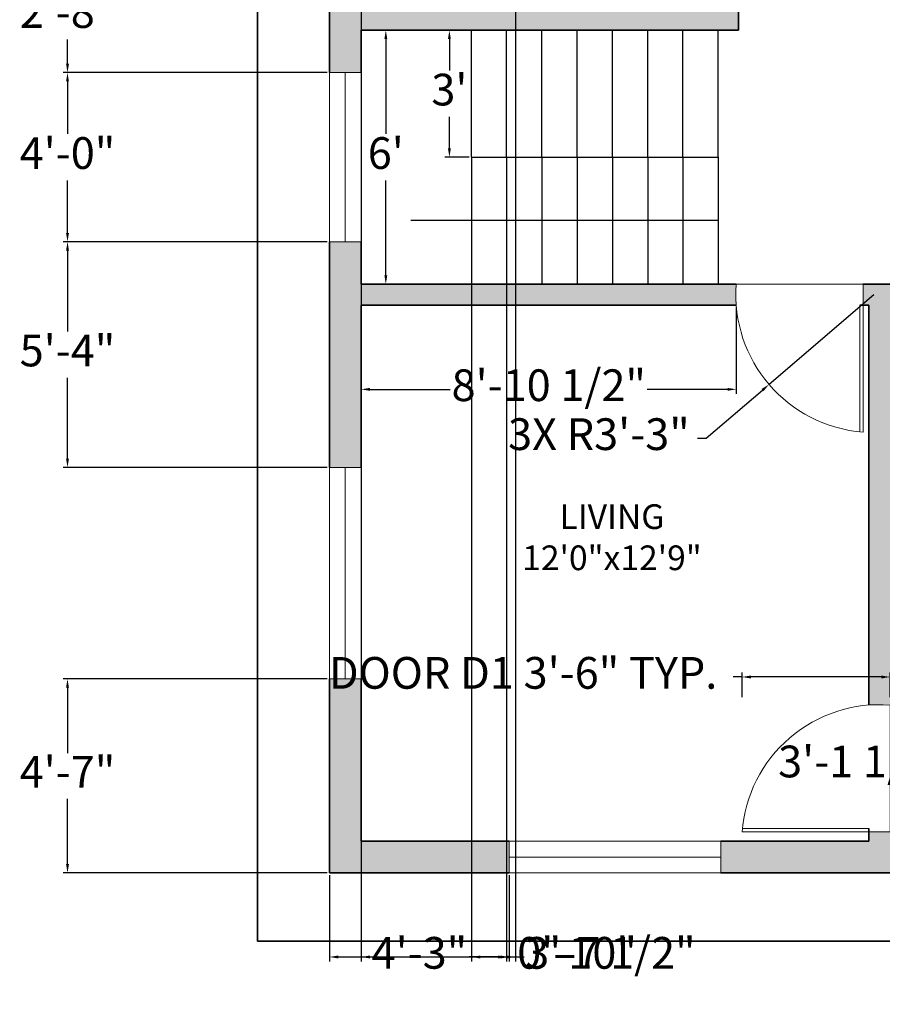
# Model space of a CAD drawing. Units: inches. Extents: x 2151 to 2709, y 3533 to 4046.
# Tile 1 of 4: x 2161 to 2406, y 3533 to 3812. Entities that reach past the tile are written whole.
import ezdxf

# ---------------------------------------------------------------- set-up
doc = ezdxf.new("R2010")
doc.units = ezdxf.units.IN
for name, color, linetype, lineweight in [('A-ANNO-DIMS', 2, 'Continuous', 18), ('A-ANNO-TTLB', 7, 'Continuous', 35), ('A-AREA-IDEN', 7, 'Continuous', 25), ('A-DOOR', 3, 'Continuous', 18), ('A-FLOR-STRS', 7, 'Continuous', 25), ('A-GLAZ', 4, 'Continuous', 18), ('A-WALL', 7, 'Continuous', 35)]:
    doc.layers.add(name, color=color, linetype=linetype, lineweight=lineweight)
doc.layers.add('A-WALL-PATT', color=18, linetype='Continuous', lineweight=13, true_color=0x000000)
doc.styles.get("Standard").update_dxf_attribs({"font": 'arial.ttf'})
doc.dimstyles.new('ISO-25', dxfattribs={"dimtxt": 9, "dimasz": 2.5, "dimexe": 1.25, "dimexo": 0.625, "dimgap": 2, "dimtad": 0, "dimtih": 1, "dimtoh": 1, "dimdec": 1, "dimlunit": 4, "dimtxsty": 'Standard', "dimcen": 2.5, "dimadec": 0, "dimazin": 0, "dimtfac": 0.5, "dimtdec": 1, "dimtmove": 0, "dimatfit": 3, "dimfxl": 1, "dimarcsym": 0})

# ---------------------------------------------------------------- blocks, each defined once
blk = doc.blocks.new('*D4')
at = {"layer": 'A-ANNO-DIMS', "color": 0, "lineweight": -2, "transparency": 16777216}
for p, q in [((2288.46, 3809.17), (2281.59, 3809.17)), ((2282.84, 3806.67), (2282.84, 3797.76)), ((2282.84, 3775.67), (2282.84, 3784.57)), ((2288.46, 3773.17), (2281.59, 3773.17))]:
    blk.add_line(p, q, dxfattribs=at)
at = {"layer": 'A-ANNO-DIMS', "color": 0, "transparency": 16777216}
for points in [[(2282.43, 3806.67), (2283.26, 3806.67), (2282.84, 3809.17)], [(2282.43, 3775.67), (2283.26, 3775.67), (2282.84, 3773.17)]]:
    blk.add_solid(points, dxfattribs=at)
at = {"layer": 'Defpoints', "color": 0, "transparency": 16777216}
for p in [(2289.08, 3809.17), (2282.84, 3773.17), (2289.08, 3773.17)]:
    blk.add_point(p, dxfattribs=at)
at = {"layer": 'A-ANNO-DIMS', "color": 0, "transparency": 16777216, "insert": (2282.84, 3791.17), "char_height": 9, "attachment_point": 5}
blk.add_mtext("3'", dxfattribs=at)
blk = doc.blocks.new('*D5')
at = {"layer": 'A-ANNO-DIMS', "color": 0, "lineweight": -2, "transparency": 16777216}
for p, q in [((2258.46, 3809.17), (2266.06, 3809.17)), ((2264.81, 3806.67), (2264.81, 3779.76)), ((2264.81, 3739.67), (2264.81, 3766.57)), ((2258.46, 3737.17), (2266.06, 3737.17))]:
    blk.add_line(p, q, dxfattribs=at)
at = {"layer": 'A-ANNO-DIMS', "color": 0, "transparency": 16777216}
for points in [[(2264.4, 3806.67), (2265.23, 3806.67), (2264.81, 3809.17)], [(2264.4, 3739.67), (2265.23, 3739.67), (2264.81, 3737.17)]]:
    blk.add_solid(points, dxfattribs=at)
at = {"layer": 'Defpoints', "color": 0, "transparency": 16777216}
for p in [(2257.83, 3809.17), (2264.81, 3809.17), (2257.83, 3737.17)]:
    blk.add_point(p, dxfattribs=at)
at = {"layer": 'A-ANNO-DIMS', "color": 0, "transparency": 16777216, "insert": (2264.81, 3773.17), "char_height": 9, "attachment_point": 5}
blk.add_mtext("6'", dxfattribs=at)
blk = doc.blocks.new('WIN-60IN')
for p, q in [((0, 9), (0, 0)), ((0, 9), (60, 9)), ((60, 9), (60, 0)), ((0, 4.5), (60, 4.5)), ((0, 0), (60, 0))]:
    blk.add_line(p, q)
blk = doc.blocks.new('DOOR-SWING-36IN')
for p, q in [((0, 6), (0, 42)), ((1, 6), (1, 41.91)), ((0, 6), (0, 0)), ((0, 0), (36, 0))]:
    blk.add_line(p, q)
blk.add_arc((-3, 3), 39.12, 355.6013, 85.6013)
blk = doc.blocks.new('*D17')
at = {"layer": 'A-ANNO-DIMS', "color": 0, "lineweight": -2, "transparency": 16777216}
for p, q in [((2365.83, 3625.73), (2363.33, 3625.73)), ((2365.83, 3620.05), (2365.83, 3626.98)), ((2405.33, 3625.73), (2368.33, 3625.73)), ((2407.83, 3620.05), (2407.83, 3626.98))]:
    blk.add_line(p, q, dxfattribs=at)
at = {"layer": 'A-ANNO-DIMS', "color": 0, "transparency": 16777216}
for points in [[(2368.33, 3626.14), (2368.33, 3625.31), (2365.83, 3625.73)], [(2405.33, 3626.14), (2405.33, 3625.31), (2407.83, 3625.73)]]:
    blk.add_solid(points, dxfattribs=at)
at = {"layer": 'Defpoints', "color": 0, "transparency": 16777216}
for p in [(2365.83, 3625.73), (2365.83, 3619.43), (2407.83, 3619.43)]:
    blk.add_point(p, dxfattribs=at)
at = {"layer": 'A-ANNO-DIMS', "color": 0, "transparency": 16777216, "insert": (2303.74, 3625.73), "char_height": 9, "attachment_point": 5}
blk.add_mtext('DOOR D1 3\'-6" TYP.', dxfattribs=at)
blk = doc.blocks.new('*D18')
at = {"layer": 'A-ANNO-DIMS', "color": 0, "lineweight": -2, "transparency": 16777216}
for p, q in [((2408.46, 3619.43), (2415.38, 3619.43)), ((2414.13, 3616.93), (2414.13, 3607.26)), ((2414.13, 3584.27), (2414.13, 3593.94)), ((2408.46, 3581.77), (2415.38, 3581.77))]:
    blk.add_line(p, q, dxfattribs=at)
at = {"layer": 'A-ANNO-DIMS', "color": 0, "transparency": 16777216}
for points in [[(2413.71, 3616.93), (2414.55, 3616.93), (2414.13, 3619.43)], [(2413.71, 3584.27), (2414.55, 3584.27), (2414.13, 3581.77)]]:
    blk.add_solid(points, dxfattribs=at)
at = {"layer": 'Defpoints', "color": 0, "transparency": 16777216}
for p in [(2407.83, 3619.43), (2414.13, 3619.43), (2407.83, 3581.77)]:
    blk.add_point(p, dxfattribs=at)
at = {"layer": 'A-ANNO-DIMS', "color": 0, "transparency": 16777216, "insert": (2414.13, 3600.6), "char_height": 9, "attachment_point": 5}
blk.add_mtext('3\'-1 1/2" TYP.', dxfattribs=at)
blk = doc.blocks.new('*D32')
at = {"layer": 'A-ANNO-DIMS', "color": 0, "lineweight": -2, "transparency": 16777216}
for p, q in [((2248.21, 3625.17), (2173.29, 3625.17)), ((2174.54, 3622.67), (2174.54, 3604.17)), ((2174.54, 3572.67), (2174.54, 3591.17)), ((2248.21, 3570.17), (2173.29, 3570.17))]:
    blk.add_line(p, q, dxfattribs=at)
at = {"layer": 'A-ANNO-DIMS', "color": 0, "transparency": 16777216}
for points in [[(2174.13, 3622.67), (2174.96, 3622.67), (2174.54, 3625.17)], [(2174.13, 3572.67), (2174.96, 3572.67), (2174.54, 3570.17)]]:
    blk.add_solid(points, dxfattribs=at)
at = {"layer": 'Defpoints', "color": 0, "transparency": 16777216}
for p in [(2174.54, 3625.17), (2248.83, 3625.17), (2248.83, 3570.17)]:
    blk.add_point(p, dxfattribs=at)
at = {"layer": 'A-ANNO-DIMS', "color": 0, "transparency": 16777216, "insert": (2174.54, 3597.67), "char_height": 9, "attachment_point": 5}
blk.add_mtext('4\'-7"', dxfattribs=at)
blk = doc.blocks.new('*D33')
at = {"layer": 'A-ANNO-DIMS', "color": 0, "lineweight": -2, "transparency": 16777216}
for p, q in [((2248.83, 3569.54), (2248.83, 3545.07)), ((2299.83, 3569.54), (2299.83, 3545.07)), ((2251.33, 3546.32), (2260.19, 3546.32)), ((2297.33, 3546.32), (2288.47, 3546.32))]:
    blk.add_line(p, q, dxfattribs=at)
at = {"layer": 'A-ANNO-DIMS', "color": 0, "transparency": 16777216}
for points in [[(2251.33, 3546.73), (2251.33, 3545.9), (2248.83, 3546.32)], [(2297.33, 3546.73), (2297.33, 3545.9), (2299.83, 3546.32)]]:
    blk.add_solid(points, dxfattribs=at)
at = {"layer": 'Defpoints', "color": 0, "transparency": 16777216}
for p in [(2248.83, 3570.17), (2299.83, 3570.17), (2299.83, 3546.32)]:
    blk.add_point(p, dxfattribs=at)
at = {"layer": 'A-ANNO-DIMS', "color": 0, "transparency": 16777216, "insert": (2274.33, 3546.32), "char_height": 9, "attachment_point": 5}
blk.add_mtext('4\'-3"', dxfattribs=at)
blk = doc.blocks.new('*D35')
at = {"layer": 'A-ANNO-DIMS', "color": 0, "lineweight": -2, "transparency": 16777216}
for p, q in [((2248.21, 3797.17), (2173.29, 3797.17)), ((2174.54, 3794.67), (2174.54, 3779.76)), ((2174.54, 3751.67), (2174.54, 3766.57)), ((2248.21, 3749.17), (2173.29, 3749.17))]:
    blk.add_line(p, q, dxfattribs=at)
at = {"layer": 'A-ANNO-DIMS', "color": 0, "transparency": 16777216}
for points in [[(2174.13, 3794.67), (2174.96, 3794.67), (2174.54, 3797.17)], [(2174.13, 3751.67), (2174.96, 3751.67), (2174.54, 3749.17)]]:
    blk.add_solid(points, dxfattribs=at)
at = {"layer": 'Defpoints', "color": 0, "transparency": 16777216}
for p in [(2174.54, 3797.17), (2248.83, 3797.17), (2248.83, 3749.17)]:
    blk.add_point(p, dxfattribs=at)
at = {"layer": 'A-ANNO-DIMS', "color": 0, "transparency": 16777216, "insert": (2174.54, 3773.17), "char_height": 9, "attachment_point": 5}
blk.add_mtext('4\'-0"', dxfattribs=at)
blk = doc.blocks.new('*D36')
at = {"layer": 'A-ANNO-DIMS', "color": 0, "lineweight": -2, "transparency": 16777216}
for p, q in [((2248.21, 3829.17), (2173.29, 3829.17)), ((2174.54, 3826.67), (2174.54, 3819.76)), ((2174.54, 3799.67), (2174.54, 3806.57)), ((2248.21, 3797.17), (2173.29, 3797.17))]:
    blk.add_line(p, q, dxfattribs=at)
at = {"layer": 'A-ANNO-DIMS', "color": 0, "transparency": 16777216}
for points in [[(2174.13, 3826.67), (2174.96, 3826.67), (2174.54, 3829.17)], [(2174.13, 3799.67), (2174.96, 3799.67), (2174.54, 3797.17)]]:
    blk.add_solid(points, dxfattribs=at)
at = {"layer": 'Defpoints', "color": 0, "transparency": 16777216}
for p in [(2174.54, 3829.17), (2248.83, 3829.17), (2248.83, 3797.17)]:
    blk.add_point(p, dxfattribs=at)
at = {"layer": 'A-ANNO-DIMS', "color": 0, "transparency": 16777216, "insert": (2174.54, 3813.17), "char_height": 9, "attachment_point": 5}
blk.add_mtext('2\'-8"', dxfattribs=at)
blk = doc.blocks.new('*D37')
at = {"layer": 'A-ANNO-DIMS', "color": 0, "lineweight": -2, "transparency": 16777216}
for p, q in [((2248.21, 3749.17), (2173.29, 3749.17)), ((2174.54, 3746.67), (2174.54, 3723.74)), ((2174.54, 3687.67), (2174.54, 3710.59)), ((2248.21, 3685.17), (2173.29, 3685.17))]:
    blk.add_line(p, q, dxfattribs=at)
at = {"layer": 'A-ANNO-DIMS', "color": 0, "transparency": 16777216}
for points in [[(2174.13, 3746.67), (2174.96, 3746.67), (2174.54, 3749.17)], [(2174.13, 3687.67), (2174.96, 3687.67), (2174.54, 3685.17)]]:
    blk.add_solid(points, dxfattribs=at)
at = {"layer": 'Defpoints', "color": 0, "transparency": 16777216}
for p in [(2174.54, 3749.17), (2248.83, 3749.17), (2248.83, 3685.17)]:
    blk.add_point(p, dxfattribs=at)
at = {"layer": 'A-ANNO-DIMS', "color": 0, "transparency": 16777216, "insert": (2174.54, 3717.17), "char_height": 9, "attachment_point": 5}
blk.add_mtext('5\'-4"', dxfattribs=at)
blk = doc.blocks.new('*D41')
at = {"layer": 'A-ANNO-DIMS', "color": 0, "lineweight": -2, "transparency": 16777216}
for p, q in [((2257.83, 3992.54), (2257.83, 3545.07)), ((2301.55, 3992.54), (2301.55, 3545.07)), ((2260.33, 3546.32), (2299.05, 3546.32)), ((2301.55, 3546.32), (2304.05, 3546.32))]:
    blk.add_line(p, q, dxfattribs=at)
at = {"layer": 'A-ANNO-DIMS', "color": 0, "transparency": 16777216}
for points in [[(2260.33, 3546.73), (2260.33, 3545.9), (2257.83, 3546.32)], [(2299.05, 3546.73), (2299.05, 3545.9), (2301.55, 3546.32)]]:
    blk.add_solid(points, dxfattribs=at)
at = {"layer": 'Defpoints', "color": 0, "transparency": 16777216}
for p in [(2257.83, 3993.17), (2301.55, 3993.17), (2301.55, 3546.32)]:
    blk.add_point(p, dxfattribs=at)
at = {"layer": 'A-ANNO-DIMS', "color": 0, "transparency": 16777216, "insert": (2328.5, 3546.32), "char_height": 9, "attachment_point": 5}
blk.add_mtext('3\'-7 1/2"', dxfattribs=at)
blk = doc.blocks.new('*D46')
at = {"layer": 'A-ANNO-DIMS', "color": 0, "lineweight": -2, "transparency": 16777216}
for p, q in [((2289.08, 3772.54), (2289.08, 3545.07)), ((2299.08, 3772.54), (2299.08, 3545.07)), ((2291.58, 3546.32), (2296.58, 3546.32)), ((2299.08, 3546.32), (2301.58, 3546.32))]:
    blk.add_line(p, q, dxfattribs=at)
at = {"layer": 'A-ANNO-DIMS', "color": 0, "transparency": 16777216}
for points in [[(2291.58, 3546.73), (2291.58, 3545.9), (2289.08, 3546.32)], [(2296.58, 3546.73), (2296.58, 3545.9), (2299.08, 3546.32)]]:
    blk.add_solid(points, dxfattribs=at)
at = {"layer": 'Defpoints', "color": 0, "transparency": 16777216}
for p in [(2289.08, 3773.17), (2299.08, 3773.17), (2299.08, 3546.32)]:
    blk.add_point(p, dxfattribs=at)
at = {"layer": 'A-ANNO-DIMS', "color": 0, "transparency": 16777216, "insert": (2319.04, 3546.32), "char_height": 9, "attachment_point": 5}
blk.add_mtext('0\'-10"', dxfattribs=at)
blk = doc.blocks.new('*D49')
at = {"layer": 'A-ANNO-DIMS', "color": 0, "lineweight": -2, "transparency": 16777216}
for p, q in [((2257.83, 3730.54), (2257.83, 3706.07)), ((2364.21, 3730.54), (2364.21, 3706.07)), ((2260.33, 3707.32), (2283.07, 3707.32)), ((2361.71, 3707.32), (2338.97, 3707.32))]:
    blk.add_line(p, q, dxfattribs=at)
at = {"layer": 'A-ANNO-DIMS', "color": 0, "transparency": 16777216}
for points in [[(2260.33, 3707.73), (2260.33, 3706.9), (2257.83, 3707.32)], [(2361.71, 3707.73), (2361.71, 3706.9), (2364.21, 3707.32)]]:
    blk.add_solid(points, dxfattribs=at)
at = {"layer": 'Defpoints', "color": 0, "transparency": 16777216}
for p in [(2257.83, 3731.17), (2364.21, 3731.17), (2257.83, 3707.32)]:
    blk.add_point(p, dxfattribs=at)
at = {"layer": 'A-ANNO-DIMS', "color": 0, "transparency": 16777216, "insert": (2311.02, 3707.32), "char_height": 9, "attachment_point": 5}
blk.add_mtext('8\'-10 1/2"', dxfattribs=at)
blk = doc.blocks.new('*D57')
at = {"layer": 'A-ANNO-DIMS', "color": 0, "lineweight": -2, "transparency": 16777216}
for p, q in [((2403.21, 3734.17), (2373.51, 3708.71)), ((2355.69, 3693.44), (2371.61, 3707.08)), ((2353.19, 3693.44), (2355.69, 3693.44))]:
    blk.add_line(p, q, dxfattribs=at)
at = {"layer": 'A-ANNO-DIMS', "color": 0, "transparency": 16777216}
blk.add_solid([(2371.34, 3707.4), (2371.88, 3706.77), (2373.51, 3708.71)], dxfattribs=at)
at = {"layer": 'Defpoints', "color": 0, "transparency": 16777216}
for p in [(2403.21, 3734.17), (2373.51, 3708.71)]:
    blk.add_point(p, dxfattribs=at)
at = {"layer": 'A-ANNO-DIMS', "color": 0, "transparency": 16777216, "insert": (2325.25, 3693.44), "char_height": 9, "attachment_point": 5}
blk.add_mtext('3X R3\'-3"', dxfattribs=at)

msp = doc.modelspace()

# ---------------------------------------------------------------- hatches: boundary and pattern name
at = {"layer": 'A-WALL-PATT'}
h = msp.add_hatch(color=256, dxfattribs=at)
h.dxf.hatch_style = 1
h.paths.add_polyline_path([(2428.83, 4002.17), (2248.83, 4002.17), (2248.83, 3969.17), (2257.83, 3969.17), (2257.83, 3993.17), (2401.83, 3993.17), (2401.83, 3873.17), (2399.81, 3873.17), (2399.81, 3867.17), (2410.61, 3867.17), (2410.61, 3873.17), (2407.83, 3873.17), (2407.83, 3993.17), (2428.83, 3993.17)])
h.paths.add_polyline_path([(2632.83, 4002.17), (2452.83, 4002.17), (2452.83, 3993.17), (2473.83, 3993.17), (2473.83, 3873.17), (2440.61, 3873.17, -0.045361), (2440.61, 3867.17), (2482.29, 3867.17), (2482.29, 3873.17), (2479.83, 3873.17), (2479.83, 3993.17), (2623.83, 3993.17), (2623.83, 3969.17), (2632.83, 3969.17)])
h.paths.add_polyline_path([(2257.83, 3897.17), (2248.83, 3897.17), (2248.83, 3853.17), (2257.83, 3853.17), (2257.83, 3867.17), (2324.99, 3867.17, -0.045361), (2324.99, 3873.17), (2257.83, 3873.17)])
h.paths.add_polyline_path([(2632.83, 3897.17), (2623.83, 3897.17), (2623.83, 3873.17), (2518.29, 3873.17, -0.038405), (2518.29, 3867.17), (2623.83, 3867.17), (2623.83, 3838.17), (2632.83, 3838.17)])
h.paths.add_polyline_path([(2364.83, 3815.17), (2364.83, 3867.17), (2365.88, 3867.17, -0.038164), (2365.88, 3873.17), (2354.99, 3873.17), (2354.99, 3867.17), (2358.83, 3867.17), (2358.83, 3815.17), (2257.83, 3815.17), (2257.83, 3829.17), (2248.83, 3829.17), (2248.83, 3797.17), (2257.83, 3797.17), (2257.83, 3809.17), (2358.83, 3809.17), (2364.83, 3809.17)])
h.paths.add_polyline_path([(2364.21, 3737.17), (2257.83, 3737.17), (2257.83, 3749.17), (2248.83, 3749.17), (2248.83, 3685.17), (2257.83, 3685.17), (2257.83, 3731.17), (2364.21, 3731.17, -0.038405)])
h.paths.add_polyline_path([(2257.83, 3625.17), (2248.83, 3625.17), (2248.83, 3570.17), (2299.83, 3570.17), (2299.83, 3579.17), (2257.83, 3579.17)])
h = msp.add_hatch(color=256, dxfattribs=at)
h.dxf.hatch_style = 1
h.paths.add_polyline_path([(2407.83, 3731.17), (2407.83, 3737.17), (2400.21, 3737.17), (2400.21, 3731.17), (2401.83, 3731.17), (2401.83, 3617.77, -0.038405), (2407.83, 3617.77), (2407.83, 3634.17), (2410.59, 3634.17), (2410.59, 3643.17), (2407.83, 3643.17)])
h.paths.add_polyline_path([(2407.83, 3579.17), (2407.83, 3581.77), (2401.83, 3581.77), (2401.83, 3579.17), (2359.83, 3579.17), (2359.83, 3570.17), (2407.83, 3570.17)])

# ---------------------------------------------------------------- linework, layer by layer
at = {"layer": 'A-ANNO-TTLB'}
msp.add_lwpolyline([(2228.43, 4045.57), (2671.96, 4045.57), (2671.96, 3550.81), (2228.43, 3550.81)], close=True, dxfattribs=at)
at = {"layer": 'A-FLOR-STRS'}
for p, q in [((2289.08, 3773.17), (2289.08, 3809.17)), ((2299.08, 3773.17), (2299.08, 3809.17)), ((2309.08, 3773.17), (2309.08, 3809.17)), ((2319.08, 3773.17), (2319.08, 3809.17)), ((2329.08, 3773.17), (2329.08, 3809.17)), ((2339.08, 3773.17), (2339.08, 3809.17)), ((2349.08, 3773.17), (2349.08, 3809.17)), ((2359.08, 3773.17), (2359.08, 3809.17)), ((2289.08, 3773.17), (2359.08, 3773.17)), ((2289.08, 3773.17), (2289.08, 3737.17)), ((2299.08, 3773.17), (2299.08, 3737.17)), ((2309.08, 3773.17), (2309.08, 3737.17)), ((2319.08, 3773.17), (2319.08, 3737.17)), ((2329.08, 3773.17), (2329.08, 3737.17)), ((2339.08, 3773.17), (2339.08, 3737.17)), ((2349.08, 3773.17), (2349.08, 3737.17)), ((2359.08, 3773.17), (2359.08, 3737.17)), ((2359.08, 3755.17), (2271.9, 3755.17))]:
    msp.add_line(p, q, dxfattribs=at)
at = {"layer": 'A-GLAZ'}
for p, q in [((2257.83, 3797.17), (2248.83, 3797.17)), ((2248.83, 3797.17), (2248.83, 3749.17)), ((2253.33, 3797.17), (2253.33, 3749.17)), ((2257.83, 3797.17), (2257.83, 3749.17)), ((2257.83, 3749.17), (2248.83, 3749.17))]:
    msp.add_line(p, q, dxfattribs=at)
at = {"layer": 'A-WALL'}
for p, q in [((2248.83, 3797.17), (2248.83, 3829.17)), ((2364.83, 3815.17), (2364.83, 3809.17)), ((2257.83, 3809.17), (2358.83, 3809.17)), ((2257.83, 3797.17), (2257.83, 3809.17)), ((2358.83, 3809.17), (2364.83, 3809.17)), ((2248.83, 3685.17), (2248.83, 3749.17)), ((2257.83, 3737.17), (2257.83, 3749.17)), ((2257.83, 3737.17), (2364.21, 3737.17)), ((2400.21, 3737.17), (2407.83, 3737.17)), ((2400.21, 3737.17), (2407.83, 3737.17)), ((2257.83, 3731.17), (2364.21, 3731.17)), ((2257.83, 3685.17), (2257.83, 3731.17)), ((2399.21, 3731.17), (2401.83, 3731.17)), ((2401.83, 3617.77), (2401.83, 3731.17)), ((2248.83, 3570.17), (2248.83, 3625.17)), ((2257.83, 3579.17), (2257.83, 3625.17)), ((2401.83, 3579.17), (2401.83, 3582.77)), ((2299.83, 3579.17), (2257.83, 3579.17)), ((2401.83, 3579.17), (2359.83, 3579.17)), ((2299.83, 3570.17), (2248.83, 3570.17)), ((2632.83, 3570.17), (2359.83, 3570.17))]:
    msp.add_line(p, q, dxfattribs=at)

# ---------------------------------------------------------------- block references
at = {"layer": 'A-DOOR'}
for p, rotation in [((2400.21, 3737.17), 180), ((2407.83, 3581.77), 89.99999999999812)]:
    msp.add_blockref('DOOR-SWING-36IN', p, dxfattribs=dict(at, rotation=rotation))
at = {"layer": 'A-GLAZ', "rotation": 89.9999999999925}
msp.add_blockref('WIN-60IN', (2257.83, 3625.17), dxfattribs=at)
at = {"layer": 'A-GLAZ'}
msp.add_blockref('WIN-60IN', (2299.83, 3570.17), dxfattribs=at)

# ---------------------------------------------------------------- texts
at = {"layer": 'A-AREA-IDEN', "insert": (2294.92, 3674.71), "char_height": 7, "attachment_point": 1}
msp.add_mtext_dynamic_manual_height_columns('\\pxqc;{\\fArial|b1|i0|c0|p34;LIVING\\P12\'0"x12\'9"}', width=68.0562, gutter_width=12.5, heights=[0], dxfattribs=at)

# ---------------------------------------------------------------- dimensions: what is measured, and where the dimension line sits
at = {"layer": 'A-ANNO-DIMS'}
for base, p1, p2, picture, middle in [((2301.55, 3546.32), (2257.83, 3993.17), (2301.55, 3993.17), '*D41', (2328.5, 3546.32)), ((2299.08, 3546.32), (2289.08, 3773.17), (2299.08, 3773.17), '*D46', (2319.04, 3546.32)), ((2299.83, 3546.32), (2248.83, 3570.17), (2299.83, 3570.17), '*D33', (2274.33, 3546.32))]:
    dim = msp.add_linear_dim(base=base, p1=p1, p2=p2, dimstyle='ISO-25', override={"dimdec": 1, "dimlfac": 1, "dimrnd": 0, "dimzin": 1, "dimdsep": 46, "dimlunit": 4, "dimfrac": 2}, dxfattribs=at)
    dim.commit()
    dim.dimension.update_dxf_attribs({"geometry": picture, "text_midpoint": middle})
for base, p1, p2, angle, override, picture, middle in [((2174.54, 3829.17), (2248.83, 3797.17), (2248.83, 3829.17), 90, {"dimdec": 1, "dimlfac": 1, "dimrnd": 0, "dimzin": 1, "dimdsep": 46, "dimlunit": 4, "dimfrac": 2}, '*D36', (2174.54, 3813.17)), ((2264.81, 3809.17), (2257.83, 3737.17), (2257.83, 3809.17), 90, {"dimclrd": 0, "dimclre": 0, "dimclrt": 0}, '*D5', (2264.81, 3773.17)), ((2174.54, 3797.17), (2248.83, 3749.17), (2248.83, 3797.17), 90, {"dimdec": 1, "dimlfac": 1, "dimrnd": 0, "dimzin": 1, "dimdsep": 46, "dimlunit": 4, "dimfrac": 2}, '*D35', (2174.54, 3773.17)), ((2174.54, 3749.17), (2248.83, 3685.17), (2248.83, 3749.17), 90, {"dimdec": 1, "dimlfac": 1, "dimrnd": 0, "dimzin": 1, "dimdsep": 46, "dimlunit": 4, "dimfrac": 2}, '*D37', (2174.54, 3717.17)), ((2257.83, 3707.32), (2364.21, 3731.17), (2257.83, 3731.17), 180, {"dimdec": 1, "dimlfac": 1, "dimrnd": 0, "dimzin": 1, "dimdsep": 46, "dimlunit": 4, "dimfrac": 2}, '*D49', (2311.02, 3707.32)), ((2174.54, 3625.17), (2248.83, 3570.17), (2248.83, 3625.17), 90, {"dimdec": 1, "dimlfac": 1, "dimrnd": 0, "dimzin": 1, "dimdsep": 46, "dimlunit": 4, "dimfrac": 2}, '*D32', (2174.54, 3597.67))]:
    dim = msp.add_linear_dim(base=base, p1=p1, p2=p2, angle=angle, dimstyle='ISO-25', override=override, dxfattribs=at)
    dim.commit()
    dim.dimension.update_dxf_attribs({"geometry": picture, "text_midpoint": middle})
dim = msp.add_aligned_dim(p1=(2289.08, 3809.17), p2=(2289.08, 3773.17), distance=-6.24, dimstyle='ISO-25', override={"dimclrd": 0, "dimclre": 0, "dimclrt": 0}, dxfattribs=at)
dim.commit()
dim.dimension.update_dxf_attribs({"geometry": '*D4', "text_midpoint": (2282.84, 3791.17)})
dim = msp.add_radius_dim(center=(2403.21, 3734.17), mpoint=(2373.51, 3708.71), text='3X <>', dimstyle='ISO-25', override={"dimdec": 1, "dimlfac": 1, "dimrnd": 0, "dimzin": 1, "dimdsep": 46, "dimlunit": 4, "dimfrac": 2}, dxfattribs=at)
dim.commit()
dim.dimension.update_dxf_attribs({"geometry": '*D57', "text_midpoint": (2325.25, 3693.44), "dimtype": 164})
for base, p1, p2, angle, text, picture, middle in [((2365.83, 3625.73), (2407.83, 3619.43), (2365.83, 3619.43), 180, 'DOOR D1 <> TYP.', '*D17', (2303.74, 3625.73)), ((2414.13, 3619.43), (2407.83, 3581.77), (2407.83, 3619.43), 90, '<> TYP.', '*D18', (2414.13, 3600.6))]:
    dim = msp.add_linear_dim(base=base, p1=p1, p2=p2, angle=angle, text=text, dimstyle='ISO-25', override={"dimdec": 1, "dimlfac": 1, "dimrnd": 0, "dimzin": 1, "dimdsep": 46, "dimlunit": 4, "dimfrac": 2}, dxfattribs=at)
    dim.commit()
    dim.dimension.update_dxf_attribs({"geometry": picture, "text_midpoint": middle})

doc.saveas('drawing.dxf')
